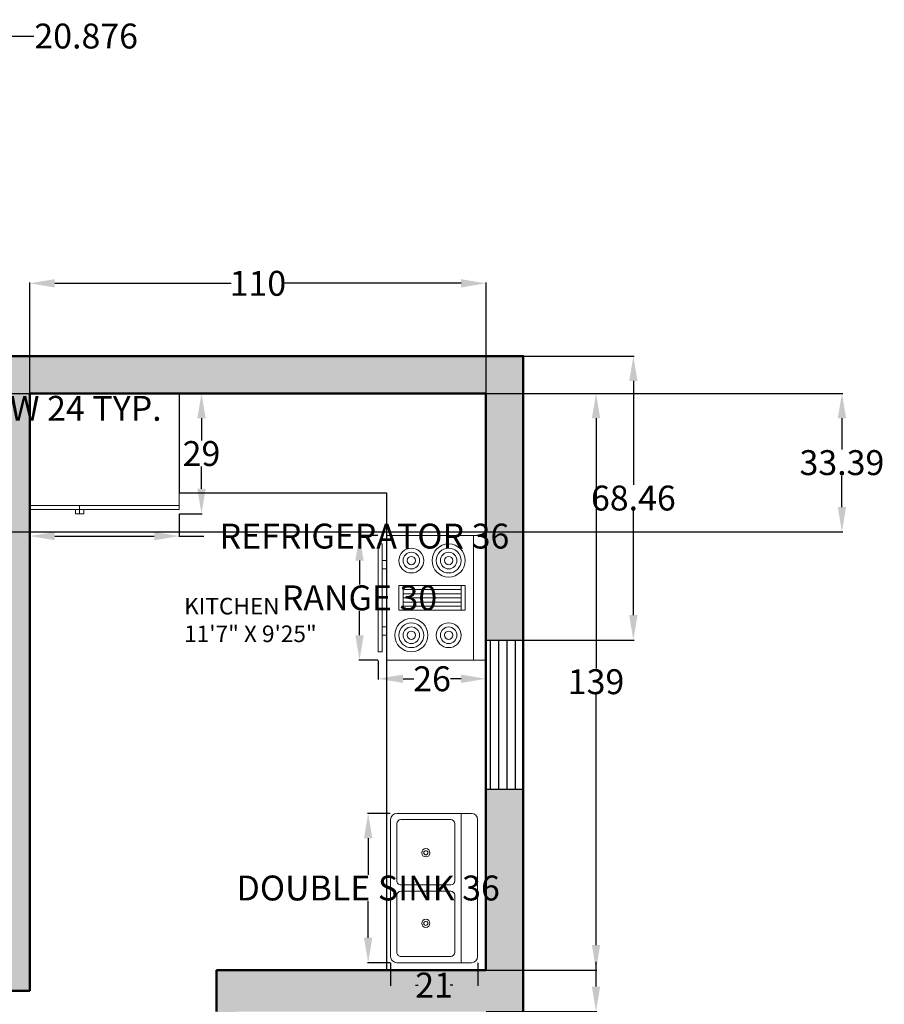
# Model space of a CAD drawing. Units: inches. Extents: x -40 to 482, y -490 to 102.
# Tile 4 of 4: x 273 to 482, y -136 to 102. Entities that reach past the tile are written whole.
import ezdxf

# ---------------------------------------------------------------- set-up
doc = ezdxf.new("R2010")
doc.units = ezdxf.units.IN
doc.header["$MEASUREMENT"] = 0
for name, color, linetype, lineweight in [('A-ANNO-DIMS', 2, 'Continuous', 18), ('A-AREA-IDEN', 7, 'Continuous', 18), ('A-EQPM', 9, 'Continuous', 18), ('A-FLOR-CASE', 32, 'Continuous', 25), ('A-FLOR-FIXT', 9, 'Continuous', 18), ('A-WALL', 7, 'Continuous', 50), ('A-WALL-PATT', 251, 'Continuous', 13), ('WINDOW', 151, 'Continuous', 25)]:
    doc.layers.add(name, color=color, linetype=linetype, lineweight=lineweight)
doc.styles.get("Standard").update_dxf_attribs({"font": 'arial.ttf'})
doc.dimstyles.get("Standard").update_dxf_attribs({"dimtxt": 6, "dimasz": 6, "dimexe": 0.18, "dimexo": 0.0625, "dimgap": 0.09, "dimtad": 0, "dimtih": 1, "dimtoh": 1, "dimdec": 3, "dimzin": 0, "dimdsep": 46, "dimlunit": 4, "dimtxsty": 'Standard', "dimcen": 0.09, "dimadec": 0, "dimazin": 0, "dimtfac": 1, "dimtdec": 3, "dimtofl": 0, "dimtmove": 0, "dimatfit": 3, "dimfxl": 1, "dimtolj": 1, "dimtzin": 0, "dimarcsym": 0})

# ---------------------------------------------------------------- blocks, each defined once
blk = doc.blocks.new('WINDOW')
for p, q in [((0, 0), (36, 0)), ((0, -9), (0, 0)), ((36, 0), (36, -9)), ((0, -2), (36, -2)), ((0, -4), (36, -4)), ((0, -6), (36, -6)), ((0, -8), (36, -8)), ((36, -9), (0, -9))]:
    blk.add_line(p, q)
blk = doc.blocks.new('Sink-double - 36 in top')
for p, q in [((-18, -4), (18, -4)), ((-0.75, -18.5), (-0.75, -6.5)), ((0.75, -6.5), (0.75, -18.5))]:
    blk.add_line(p, q)
for points in [[(-16.5, 0), (16.5, 0)], [(-18, -19.5), (-18, -1.5)], [(18, -1.5), (18, -19.5)], [(-16.5, -18.5), (-16.5, -6.5)], [(-15.5, -5.5), (-1.75, -5.5)], [(1.75, -5.5), (15.5, -5.5)], [(16.5, -6.5), (16.5, -18.5)], [(16.5, -21), (-16.5, -21)], [(-1.75, -19.5), (-15.5, -19.5)], [(15.5, -19.5), (1.75, -19.5)]]:
    blk.add_lwpolyline(points)
for centre, radius in [((-8.5, -12.5), 1), ((8.5, -12.5), 1), ((-8.5, -12.5), 0.5), ((8.5, -12.5), 0.5)]:
    blk.add_circle(centre, radius)
for centre, radius, start, end in [((-16.5, -1.5), 1.5, 90, 180), ((16.5, -1.5), 1.5, 0, 90), ((-15.5, -6.5), 1, 90, 180), ((-1.75, -6.5), 1, 0, 90), ((1.75, -6.5), 1, 90, 180), ((15.5, -6.5), 1, 0, 90), ((-15.5, -18.5), 1, 180, 270), ((-1.75, -18.5), 1, 270, 0), ((1.75, -18.5), 1, 180, 270), ((15.5, -18.5), 1, 270, 0), ((-16.5, -19.5), 1.5, 180, 270), ((16.5, -19.5), 1.5, 270, 0)]:
    blk.add_arc(centre, radius, start, end)
blk = doc.blocks.new('Range-Oven - 30 in top')
for p, q in [((0, -3), (30, -3)), ((12, -6), (18, -6)), ((13, -20), (13, -6)), ((14, -6), (14, -20)), ((15, -20), (15, -6)), ((16, -6), (16, -20)), ((17, -20), (17, -6)), ((18, -20), (12, -20)), ((6, -24), (6, -25)), ((8, -25), (8, -24)), ((22, -25), (22, -24)), ((24, -24), (24, -25))]:
    blk.add_line(p, q)
for points in [[(0, -24), (0, 0), (30, 0), (30, -24)], [(12, -21), (12, -5), (18, -5), (18, -21)], [(2, -26), (2, -25), (28, -25), (28, -26)]]:
    blk.add_lwpolyline(points, close=True)
for centre, radius in [((6, -9), 4), ((6, -9), 3), ((6, -9), 2), ((24, -9), 3), ((24, -9), 2), ((6, -9), 1), ((24, -9), 1), ((24, -18), 4), ((6, -18), 3), ((6, -18), 2), ((24, -18), 3), ((24, -18), 2), ((6, -18), 1), ((24, -18), 1)]:
    blk.add_circle(centre, radius)
blk = doc.blocks.new('Refrigerator-2 door - 36 in top')
for p, q in [((0, -26.999999), (36, -26.999999)), ((11, -27.999999), (11, -28.999999)), ((12, -26.999999), (12, -28.999999)), ((13, -28.999999), (13, -27.999999)), ((11, -28.999999), (13, -28.999999))]:
    blk.add_line(p, q)
blk.add_lwpolyline([(0, -27.999999), (0, 0), (36, 0), (36, -27.999999)], close=True)
blk = doc.blocks.new('*D26')
at = {"layer": 'A-ANNO-DIMS', "color": 0, "lineweight": -2, "transparency": 16777216}
for p, q in [((211.37, 11.43), (211.37, 7.71)), ((235.37, 11.43), (235.37, 7.71)), ((217.37, 7.89), (229.37, 7.89)), ((235.37, 7.89), (241.37, 7.89))]:
    blk.add_line(p, q, dxfattribs=at)
at = {"layer": 'A-ANNO-DIMS', "color": 0, "transparency": 16777216}
for points in [[(217.37, 8.89), (217.37, 6.89), (211.37, 7.89)], [(229.37, 8.89), (229.37, 6.89), (235.37, 7.89)]]:
    blk.add_solid(points, dxfattribs=at)
at = {"layer": 'Defpoints', "color": 0, "transparency": 16777216}
for p in [(211.37, 11.49), (235.37, 11.49), (235.37, 7.89)]:
    blk.add_point(p, dxfattribs=at)
at = {"layer": 'A-ANNO-DIMS', "color": 0, "transparency": 16777216, "insert": (275.73, 7.89), "char_height": 6, "attachment_point": 5}
blk.add_mtext('\\A1;WINDOW 24 TYP.', dxfattribs=at)
blk = doc.blocks.new('*D44')
at = {"layer": 'A-ANNO-DIMS', "color": 0, "lineweight": -2, "transparency": 16777216}
for p, q in [((362.78, -89.74), (357.27, -89.74)), ((357.45, -95.74), (357.45, -104.55)), ((357.45, -119.74), (357.45, -110.94)), ((362.78, -125.74), (357.27, -125.74))]:
    blk.add_line(p, q, dxfattribs=at)
at = {"layer": 'A-ANNO-DIMS', "color": 0, "transparency": 16777216}
for points in [[(356.45, -95.74), (358.45, -95.74), (357.45, -89.74)], [(356.45, -119.74), (358.45, -119.74), (357.45, -125.74)]]:
    blk.add_solid(points, dxfattribs=at)
at = {"layer": 'Defpoints', "color": 0, "transparency": 16777216}
for p in [(362.85, -89.74), (357.45, -125.74), (362.85, -125.74)]:
    blk.add_point(p, dxfattribs=at)
at = {"layer": 'A-ANNO-DIMS', "color": 0, "transparency": 16777216, "insert": (357.45, -107.74), "char_height": 6, "attachment_point": 5}
blk.add_mtext('\\A1;DOUBLE SINK 36', dxfattribs=at)
blk = doc.blocks.new('*D45')
at = {"layer": 'A-ANNO-DIMS', "color": 0, "lineweight": -2, "transparency": 16777216}
for p, q in [((362.85, -125.81), (362.85, -131.32)), ((383.85, -125.81), (383.85, -131.32)), ((368.85, -131.14), (369.49, -131.14)), ((377.85, -131.14), (377.21, -131.14))]:
    blk.add_line(p, q, dxfattribs=at)
at = {"layer": 'A-ANNO-DIMS', "color": 0, "transparency": 16777216}
for points in [[(368.85, -130.14), (368.85, -132.14), (362.85, -131.14)], [(377.85, -130.14), (377.85, -132.14), (383.85, -131.14)]]:
    blk.add_solid(points, dxfattribs=at)
at = {"layer": 'Defpoints', "color": 0, "transparency": 16777216}
for p in [(362.85, -125.74), (383.85, -125.74), (383.85, -131.14)]:
    blk.add_point(p, dxfattribs=at)
at = {"layer": 'A-ANNO-DIMS', "color": 0, "transparency": 16777216, "insert": (373.35, -131.14), "char_height": 6, "attachment_point": 5}
blk.add_mtext('\\A1;21', dxfattribs=at)
blk = doc.blocks.new('*D46')
at = {"layer": 'A-ANNO-DIMS', "color": 0, "lineweight": -2, "transparency": 16777216}
for p, q in [((359.79, -22.8), (355.18, -22.8)), ((355.36, -28.8), (355.36, -34.61)), ((355.36, -46.8), (355.36, -41)), ((359.79, -52.8), (355.18, -52.8))]:
    blk.add_line(p, q, dxfattribs=at)
at = {"layer": 'A-ANNO-DIMS', "color": 0, "transparency": 16777216}
for points in [[(354.36, -28.8), (356.36, -28.8), (355.36, -22.8)], [(354.36, -46.8), (356.36, -46.8), (355.36, -52.8)]]:
    blk.add_solid(points, dxfattribs=at)
at = {"layer": 'Defpoints', "color": 0, "transparency": 16777216}
for p in [(359.86, -22.8), (355.36, -52.8), (359.86, -52.8)]:
    blk.add_point(p, dxfattribs=at)
at = {"layer": 'A-ANNO-DIMS', "color": 0, "transparency": 16777216, "insert": (355.36, -37.8), "char_height": 6, "attachment_point": 5}
blk.add_mtext('\\A1;RANGE 30', dxfattribs=at)
blk = doc.blocks.new('*D47')
at = {"layer": 'A-ANNO-DIMS', "color": 0, "lineweight": -2, "transparency": 16777216}
for p, q in [((359.86, -52.87), (359.86, -57.48)), ((385.86, -52.87), (385.86, -57.48)), ((365.86, -57.3), (368.42, -57.3)), ((379.86, -57.3), (377.29, -57.3))]:
    blk.add_line(p, q, dxfattribs=at)
at = {"layer": 'A-ANNO-DIMS', "color": 0, "transparency": 16777216}
for points in [[(365.86, -56.3), (365.86, -58.3), (359.86, -57.3)], [(379.86, -56.3), (379.86, -58.3), (385.86, -57.3)]]:
    blk.add_solid(points, dxfattribs=at)
at = {"layer": 'Defpoints', "color": 0, "transparency": 16777216}
for p in [(359.86, -52.8), (385.86, -52.8), (385.86, -57.3)]:
    blk.add_point(p, dxfattribs=at)
at = {"layer": 'A-ANNO-DIMS', "color": 0, "transparency": 16777216, "insert": (372.86, -57.3), "char_height": 6, "attachment_point": 5}
blk.add_mtext('\\A1;26', dxfattribs=at)
blk = doc.blocks.new('*D48')
at = {"layer": 'A-ANNO-DIMS', "color": 0, "lineweight": -2, "transparency": 16777216}
for p, q in [((275.86, -17.57), (275.86, -23.09)), ((311.86, -17.57), (311.86, -23.09)), ((281.86, -22.91), (305.86, -22.91)), ((311.86, -22.91), (317.86, -22.91))]:
    blk.add_line(p, q, dxfattribs=at)
at = {"layer": 'A-ANNO-DIMS', "color": 0, "transparency": 16777216}
for points in [[(281.86, -21.91), (281.86, -23.91), (275.86, -22.91)], [(305.86, -21.91), (305.86, -23.91), (311.86, -22.91)]]:
    blk.add_solid(points, dxfattribs=at)
at = {"layer": 'Defpoints', "color": 0, "transparency": 16777216}
for p in [(275.86, -17.51), (311.86, -17.51), (311.86, -22.91)]:
    blk.add_point(p, dxfattribs=at)
at = {"layer": 'A-ANNO-DIMS', "color": 0, "transparency": 16777216, "insert": (356.55, -22.91), "char_height": 6, "attachment_point": 5}
blk.add_mtext('\\A1;REFRIGERATOR 36', dxfattribs=at)
blk = doc.blocks.new('*D49')
at = {"layer": 'A-ANNO-DIMS', "color": 0, "lineweight": -2, "transparency": 16777216}
for p, q in [((311.92, 11.49), (317.44, 11.49)), ((317.26, 5.49), (317.26, 0.14)), ((317.26, -11.51), (317.26, -6.16)), ((311.92, -17.51), (317.44, -17.51))]:
    blk.add_line(p, q, dxfattribs=at)
at = {"layer": 'A-ANNO-DIMS', "color": 0, "transparency": 16777216}
for points in [[(316.26, 5.49), (318.26, 5.49), (317.26, 11.49)], [(316.26, -11.51), (318.26, -11.51), (317.26, -17.51)]]:
    blk.add_solid(points, dxfattribs=at)
at = {"layer": 'Defpoints', "color": 0, "transparency": 16777216}
for p in [(311.86, 11.49), (317.26, 11.49), (311.86, -17.51)]:
    blk.add_point(p, dxfattribs=at)
at = {"layer": 'A-ANNO-DIMS', "color": 0, "transparency": 16777216, "insert": (317.26, -3.01), "char_height": 6, "attachment_point": 5}
blk.add_mtext('\\A1;29', dxfattribs=at)
blk = doc.blocks.new('*D59')
at = {"layer": 'A-ANNO-DIMS', "color": 0, "lineweight": -2, "transparency": 16777216}
for p, q in [((394.92, 20.49), (421.57, 20.49)), ((421.39, 14.49), (421.39, -10.59)), ((421.39, -41.97), (421.39, -16.89)), ((394.92, -47.97), (421.57, -47.97))]:
    blk.add_line(p, q, dxfattribs=at)
at = {"layer": 'A-ANNO-DIMS', "color": 0, "transparency": 16777216}
for points in [[(420.39, 14.49), (422.39, 14.49), (421.39, 20.49)], [(420.39, -41.97), (422.39, -41.97), (421.39, -47.97)]]:
    blk.add_solid(points, dxfattribs=at)
at = {"layer": 'Defpoints', "color": 0, "transparency": 16777216}
for p in [(394.86, 20.49), (394.86, -47.97), (421.39, -47.97)]:
    blk.add_point(p, dxfattribs=at)
at = {"layer": 'A-ANNO-DIMS', "color": 0, "transparency": 16777216, "insert": (421.39, -13.74), "char_height": 6, "attachment_point": 5}
blk.add_mtext('\\A1;68.46', dxfattribs=at)
blk = doc.blocks.new('*D60')
at = {"layer": 'A-ANNO-DIMS', "color": 0, "lineweight": -2, "transparency": 16777216}
for p, q in [((412.39, -131.51), (412.39, -125.51)), ((385.92, -137.51), (412.57, -137.51)), ((385.92, -147.35), (412.57, -147.35)), ((412.39, -153.35), (412.39, -159.35))]:
    blk.add_line(p, q, dxfattribs=at)
at = {"layer": 'A-ANNO-DIMS', "color": 0, "transparency": 16777216}
for points in [[(411.39, -131.51), (413.39, -131.51), (412.39, -137.51)], [(411.39, -153.35), (413.39, -153.35), (412.39, -147.35)]]:
    blk.add_solid(points, dxfattribs=at)
at = {"layer": 'Defpoints', "color": 0, "transparency": 16777216}
for p in [(385.86, -137.51), (385.86, -147.35), (412.39, -147.35)]:
    blk.add_point(p, dxfattribs=at)
at = {"layer": 'A-ANNO-DIMS', "color": 0, "transparency": 16777216, "insert": (412.39, -142.43), "char_height": 6, "attachment_point": 5}
blk.add_mtext('\\A1;9.845', dxfattribs=at)
blk = doc.blocks.new('*D66')
at = {"layer": 'A-ANNO-DIMS', "color": 0, "lineweight": -2, "transparency": 16777216}
for p, q in [((275.86, 11.55), (275.86, 38.2)), ((281.86, 38.02), (324.43, 38.02)), ((379.86, 38.02), (337.28, 38.02)), ((385.86, 11.55), (385.86, 38.2))]:
    blk.add_line(p, q, dxfattribs=at)
at = {"layer": 'A-ANNO-DIMS', "color": 0, "transparency": 16777216}
for points in [[(281.86, 39.02), (281.86, 37.02), (275.86, 38.02)], [(379.86, 39.02), (379.86, 37.02), (385.86, 38.02)]]:
    blk.add_solid(points, dxfattribs=at)
at = {"layer": 'Defpoints', "color": 0, "transparency": 16777216}
for p in [(385.86, 38.02), (275.86, 11.49), (385.86, 11.49)]:
    blk.add_point(p, dxfattribs=at)
at = {"layer": 'A-ANNO-DIMS', "color": 0, "transparency": 16777216, "insert": (330.86, 38.02), "char_height": 6, "attachment_point": 5}
blk.add_mtext('\\A1;110', dxfattribs=at)
blk = doc.blocks.new('*D67')
at = {"layer": 'A-ANNO-DIMS', "color": 0, "lineweight": -2, "transparency": 16777216}
for p, q in [((385.92, 11.49), (412.57, 11.49)), ((412.39, 5.49), (412.39, -54.85)), ((412.39, -121.51), (412.39, -61.16)), ((385.92, -127.51), (412.57, -127.51))]:
    blk.add_line(p, q, dxfattribs=at)
at = {"layer": 'A-ANNO-DIMS', "color": 0, "transparency": 16777216}
for points in [[(411.39, 5.49), (413.39, 5.49), (412.39, 11.49)], [(411.39, -121.51), (413.39, -121.51), (412.39, -127.51)]]:
    blk.add_solid(points, dxfattribs=at)
at = {"layer": 'Defpoints', "color": 0, "transparency": 16777216}
for p in [(385.86, 11.49), (385.86, -127.51), (412.39, -127.51)]:
    blk.add_point(p, dxfattribs=at)
at = {"layer": 'A-ANNO-DIMS', "color": 0, "transparency": 16777216, "insert": (412.39, -58.01), "char_height": 6, "attachment_point": 5}
blk.add_mtext('\\A1;139', dxfattribs=at)
blk = doc.blocks.new('*D68')
at = {"layer": 'A-ANNO-DIMS', "color": 0, "lineweight": -2, "transparency": 16777216}
for p, q in [((249.98, 11.16), (249.98, 97.81)), ((255.98, 97.63), (264.86, 97.63)), ((270.86, 11.55), (270.86, 97.81)), ((270.86, 97.63), (276.86, 97.63))]:
    blk.add_line(p, q, dxfattribs=at)
at = {"layer": 'A-ANNO-DIMS', "color": 0, "transparency": 16777216}
for points in [[(255.98, 98.63), (255.98, 96.63), (249.98, 97.63)], [(264.86, 98.63), (264.86, 96.63), (270.86, 97.63)]]:
    blk.add_solid(points, dxfattribs=at)
at = {"layer": 'Defpoints', "color": 0, "transparency": 16777216}
for p in [(270.86, 97.63), (249.98, 11.1), (270.86, 11.49)]:
    blk.add_point(p, dxfattribs=at)
at = {"layer": 'A-ANNO-DIMS', "color": 0, "transparency": 16777216, "insert": (289.45, 97.63), "char_height": 6, "attachment_point": 5}
blk.add_mtext('\\A1;20.876', dxfattribs=at)
blk = doc.blocks.new('*D69')
at = {"layer": 'A-ANNO-DIMS', "color": 0, "lineweight": -2, "transparency": 16777216}
for p, q in [((270.92, 11.49), (471.86, 11.49)), ((471.68, 5.49), (471.68, -2.05)), ((471.68, -15.9), (471.68, -8.36)), ((260.54, -21.9), (471.86, -21.9))]:
    blk.add_line(p, q, dxfattribs=at)
at = {"layer": 'A-ANNO-DIMS', "color": 0, "transparency": 16777216}
for points in [[(470.68, 5.49), (472.68, 5.49), (471.68, 11.49)], [(470.68, -15.9), (472.68, -15.9), (471.68, -21.9)]]:
    blk.add_solid(points, dxfattribs=at)
at = {"layer": 'Defpoints', "color": 0, "transparency": 16777216}
for p in [(270.86, 11.49), (471.68, 11.49), (260.48, -21.9)]:
    blk.add_point(p, dxfattribs=at)
at = {"layer": 'A-ANNO-DIMS', "color": 0, "transparency": 16777216, "insert": (471.68, -5.2), "char_height": 6, "attachment_point": 5}
blk.add_mtext('\\A1;33.39', dxfattribs=at)

msp = doc.modelspace()

# ---------------------------------------------------------------- hatches: boundary and pattern name
at = {"layer": 'A-WALL-PATT'}
h = msp.add_hatch(color=256, dxfattribs=at)
h.dxf.hatch_style = 1
h.paths.add_polyline_path([(394.8554, -267.0722), (385.8554, -267.0722), (385.8554, -280.5091), (361.8554, -280.5091), (361.8554, -285.5091), (385.8554, -285.5091), (385.8554, -344.9426), (394.8554, -344.9426)])
h.paths.add_polyline_path([(394.8554, -171.3545), (385.8554, -171.3545), (385.8554, -185.5091), (325.8554, -185.5091), (325.8554, -173.5091), (320.8554, -173.5091), (320.8554, -190.5091), (320.8554, -277.5091), (295.8554, -277.5091), (295.8554, -282.5091), (320.8554, -282.5091), (320.8554, -285.5091), (331.8554, -285.5091), (331.8554, -280.5091), (325.8554, -280.5091), (325.8554, -190.5091), (386.1154, -190.5091), (386.1154, -226.6962), (386.0363, -243.0722), (394.8554, -243.0722)])
h.paths.add_polyline_path([(394.8554, -83.9679), (385.8554, -83.9679), (385.8554, -127.5091), (320.8554, -127.5091), (320.8554, -137.5091), (320.8554, -143.5091), (325.8554, -143.5091), (325.8554, -137.5091), (385.8554, -137.5091), (385.8554, -147.3545), (394.8554, -147.3545)])
h.paths.add_polyline_path([(394.8554, 20.4909), (235.3658, 20.4909), (235.3658, 11.4909), (270.8554, 11.4909), (270.9798, 11.1006), (270.9798, 3.1006), (270.8554, -48.5091), (216.8554, -48.5091), (216.8554, -53.5091), (270.8554, -53.5091), (270.8554, -132.5091), (275.8554, -132.5091), (275.8554, 11.4909), (311.8554, 11.4909), (385.8554, 11.4909), (385.8554, -47.9679), (394.8554, -47.9679)])
h.paths.add_polyline_path([(211.3658, 20.4909), (126.5194, 20.4909), (126.5194, 11.4909), (175.8554, 11.4909), (175.8554, -84.5091), (180.8554, -84.5091), (180.8554, -53.5091), (186.8554, -53.5091), (186.8554, -48.5091), (180.8554, -48.5091), (180.8554, 11.4909), (211.3658, 11.4909)])
h.paths.add_polyline_path([(90.5194, 20.4909), (34.8554, 20.4909), (34.8554, -40.8616), (43.8554, -40.8616), (43.8554, -28.8616), (43.8554, 11.4909), (90.5194, 11.4909)])
h.paths.add_polyline_path([(43.8554, -76.8616), (34.8554, -76.8616), (34.8554, -148.5194), (43.8554, -148.5194), (43.8554, -137.5091), (180.8554, -137.5091), (180.8554, -126.5091), (175.8554, -126.5091), (175.8554, -132.5091), (43.8554, -132.5091)])
h.paths.add_polyline_path([(171.3012, -209.5091), (43.8554, -209.5091), (43.8554, -184.5194), (34.8554, -184.5194), (34.8554, -251.068), (43.8554, -251.068), (43.8554, -244.7708), (43.8554, -214.5091), (166.3012, -214.5091), (166.3012, -220.5091), (171.3012, -220.5091)])
h.paths.add_polyline_path([(171.3012, -262.5091), (166.3012, -262.5091), (166.3012, -334.5091), (43.8554, -334.5091), (43.8554, -287.068), (34.8554, -287.068), (34.8554, -459.5091), (43.8554, -459.5091), (49.8554, -459.5091), (49.8554, -450.5091), (43.8554, -450.5091), (43.8554, -339.5091), (166.3012, -339.5091), (166.3012, -450.5091), (160.3012, -450.5091), (160.3012, -459.5091), (166.3012, -459.5091), (171.3012, -459.5091), (171.3012, -450.5091), (171.3012, -445.9382), (171.3012, -410.0635), (171.3012, -407.0635), (186.7114, -407.0635), (186.7114, -401.0635), (171.3012, -401.0635)])
h.paths.add_polyline_path([(394.8554, -380.9426), (385.8554, -380.9426), (385.8554, -450.5091), (247.8554, -450.5091), (247.8554, -282.5091), (253.8554, -282.5091), (253.8554, -277.5091), (242.8554, -277.5091), (242.8554, -401.0635), (228.7114, -401.0635), (228.7114, -407.0635), (242.8554, -407.0635), (242.8554, -410.0635), (242.8554, -419.0322), (242.8554, -450.5091), (242.8554, -454.9068), (242.8554, -459.5091), (394.8554, -459.5091)])

# ---------------------------------------------------------------- linework, layer by layer
at = {"layer": 'A-FLOR-CASE'}
for p, q in [((311.8554, 11.4909), (311.8554, -12.5091)), ((311.8554, -12.5091), (361.8554, -12.5091)), ((361.8554, -12.5091), (361.8554, -127.5091))]:
    msp.add_line(p, q, dxfattribs=at)
at = {"layer": 'A-WALL'}
for p, q in [((275.8554, -132.5091), (275.8554, 11.4909)), ((275.8554, 11.4909), (385.8554, 11.4909)), ((385.8554, 11.4909), (385.8554, -127.5091)), ((320.8554, -137.5091), (320.8554, -127.5091)), ((320.8554, -127.5091), (385.8554, -127.5091)), ((270.8554, -132.5091), (275.8554, -132.5091))]:
    msp.add_line(p, q, dxfattribs=at)
msp.add_lwpolyline([(43.8554, -459.5091), (34.8554, -459.5091), (34.8554, 20.4909), (394.8554, 20.4909), (394.8554, -459.5091), (242.8554, -459.5091)], dxfattribs=at)

# ---------------------------------------------------------------- block references
at = {"layer": 'A-EQPM'}
msp.add_blockref('Refrigerator-2 door - 36 in top', (275.8554, 11.4909), dxfattribs=at)
at = {"layer": 'A-EQPM', "rotation": 270}
msp.add_blockref('Range-Oven - 30 in top', (385.8554, -22.804), dxfattribs=at)
at = {"layer": 'A-FLOR-FIXT', "rotation": 270}
msp.add_blockref('Sink-double - 36 in top', (383.8474, -107.7437), dxfattribs=at)
at = {"layer": 'WINDOW', "rotation": 270}
msp.add_blockref('WINDOW', (394.8554, -47.9679), dxfattribs=at)

# ---------------------------------------------------------------- texts
at = {"layer": 'A-AREA-IDEN', "insert": (313.0766, -37.7943), "char_height": 4, "attachment_point": 1}
msp.add_mtext_dynamic_manual_height_columns('KITCHEN\\P11\'7" X 9\'25"', width=41.765812, gutter_width=1, heights=[0], dxfattribs=at)

# ---------------------------------------------------------------- dimensions: what is measured, and where the dimension line sits
at = {"layer": 'A-ANNO-DIMS'}
for base, p1, p2, override, picture, middle in [((270.8554, 97.6321), (249.9798, 11.1006), (270.8554, 11.4909), {"dimdec": 3, "dimlfac": 1, "dimrnd": 0, "dimzin": 0, "dimdsep": 46, "dimlunit": 2}, '*D68', (289.4488, 97.6321)), ((385.8554, 38.0224), (275.8554, 11.4909), (385.8554, 11.4909), {"dimdec": 0, "dimlfac": 1, "dimrnd": 0, "dimzin": 0, "dimdsep": 46, "dimlunit": 2}, '*D66', (330.8554, 38.0224)), ((385.8554, -57.304), (359.8554, -52.804), (385.8554, -52.804), {"dimdec": 0, "dimlfac": 1, "dimrnd": 0, "dimzin": 0, "dimdsep": 46, "dimlunit": 2}, '*D47', (372.8554, -57.304)), ((383.8474, -131.1437), (362.8474, -125.7437), (383.8474, -125.7437), {"dimdec": 0, "dimlfac": 1, "dimrnd": 0, "dimzin": 0, "dimdsep": 46, "dimlunit": 2}, '*D45', (373.3474, -131.1437))]:
    dim = msp.add_linear_dim(base=base, p1=p1, p2=p2, dimstyle='Standard', override=override, dxfattribs=at)
    dim.commit()
    dim.dimension.update_dxf_attribs({"geometry": picture, "text_midpoint": middle})
for base, p1, p2, text, picture, middle in [((235.3658, 7.8909), (211.3658, 11.4909), (235.3658, 11.4909), 'WINDOW <> TYP.', '*D26', (275.7348, 7.8909)), ((311.8554, -22.9091), (275.8554, -17.5091), (311.8554, -17.5091), 'REFRIGERATOR <>', '*D48', (356.5464, -22.9091))]:
    dim = msp.add_linear_dim(base=base, p1=p1, p2=p2, text=text, dimstyle='Standard', override={"dimdec": 0, "dimlfac": 1, "dimrnd": 0, "dimzin": 0, "dimdsep": 46, "dimlunit": 2}, dxfattribs=at)
    dim.commit()
    dim.dimension.update_dxf_attribs({"geometry": picture, "text_midpoint": middle})
for base, p1, p2, angle, override, picture, middle in [((421.3869, -47.9679), (394.8554, 20.4909), (394.8554, -47.9679), 270, {"dimdec": 2, "dimlfac": 1, "dimrnd": 0, "dimzin": 0, "dimdsep": 46, "dimlunit": 2}, '*D59', (421.3869, -13.7385)), ((471.6767, 11.4909), (260.4799, -21.8994), (270.8554, 11.4909), 90, {"dimdec": 2, "dimlfac": 1, "dimrnd": 0, "dimzin": 0, "dimdsep": 46, "dimlunit": 2}, '*D69', (471.6767, -5.2042)), ((317.2554, 11.4909), (311.8554, -17.5091), (311.8554, 11.4909), 90, {"dimdec": 0, "dimlfac": 1, "dimrnd": 0, "dimzin": 0, "dimdsep": 46, "dimlunit": 2}, '*D49', (317.2554, -3.0091)), ((412.3869, -127.5091), (385.8554, 11.4909), (385.8554, -127.5091), 270, {"dimdec": 0, "dimlfac": 1, "dimrnd": 0, "dimzin": 0, "dimdsep": 46, "dimlunit": 2}, '*D67', (412.3869, -58.0091)), ((412.3869, -147.3545), (385.8554, -137.5091), (385.8554, -147.3545), 270, {"dimdec": 3, "dimlfac": 1, "dimrnd": 0, "dimzin": 0, "dimdsep": 46, "dimlunit": 2}, '*D60', (412.3869, -142.4318))]:
    dim = msp.add_linear_dim(base=base, p1=p1, p2=p2, angle=angle, dimstyle='Standard', override=override, dxfattribs=at)
    dim.commit()
    dim.dimension.update_dxf_attribs({"geometry": picture, "text_midpoint": middle})
for base, p1, p2, text, picture, middle in [((355.3554, -52.804), (359.8554, -22.804), (359.8554, -52.804), 'RANGE <>', '*D46', (355.3554, -37.804)), ((357.4474, -125.7437), (362.8474, -89.7437), (362.8474, -125.7437), 'DOUBLE SINK <>', '*D44', (357.4474, -107.7437))]:
    dim = msp.add_linear_dim(base=base, p1=p1, p2=p2, angle=270, text=text, dimstyle='Standard', override={"dimdec": 0, "dimlfac": 1, "dimrnd": 0, "dimzin": 0, "dimdsep": 46, "dimlunit": 2}, dxfattribs=at)
    dim.commit()
    dim.dimension.update_dxf_attribs({"geometry": picture, "text_midpoint": middle})

doc.saveas('drawing.dxf')
